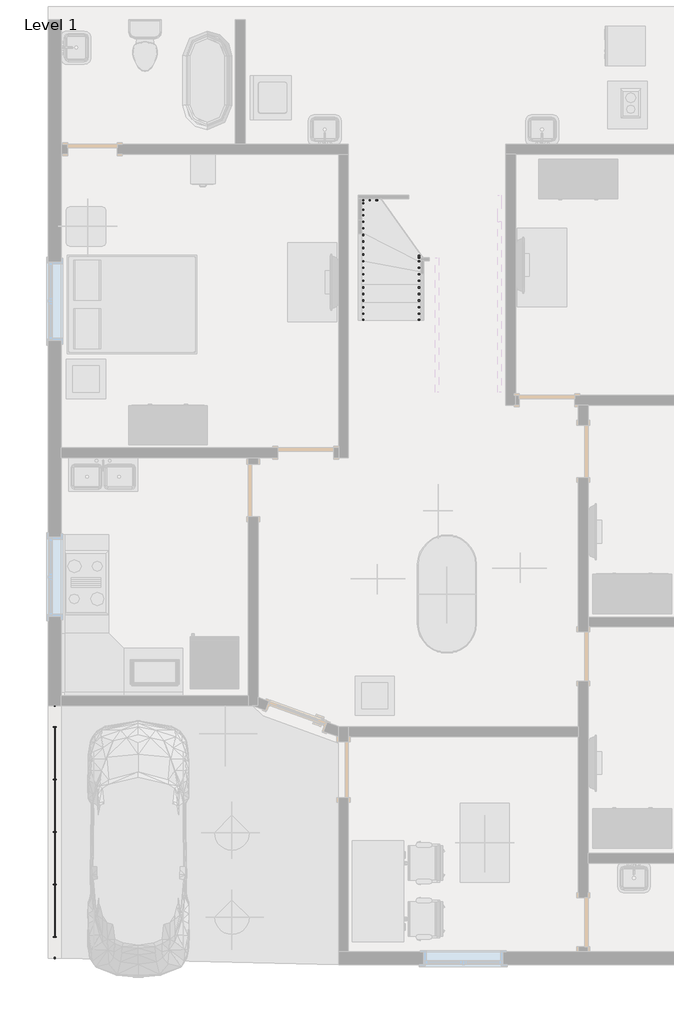
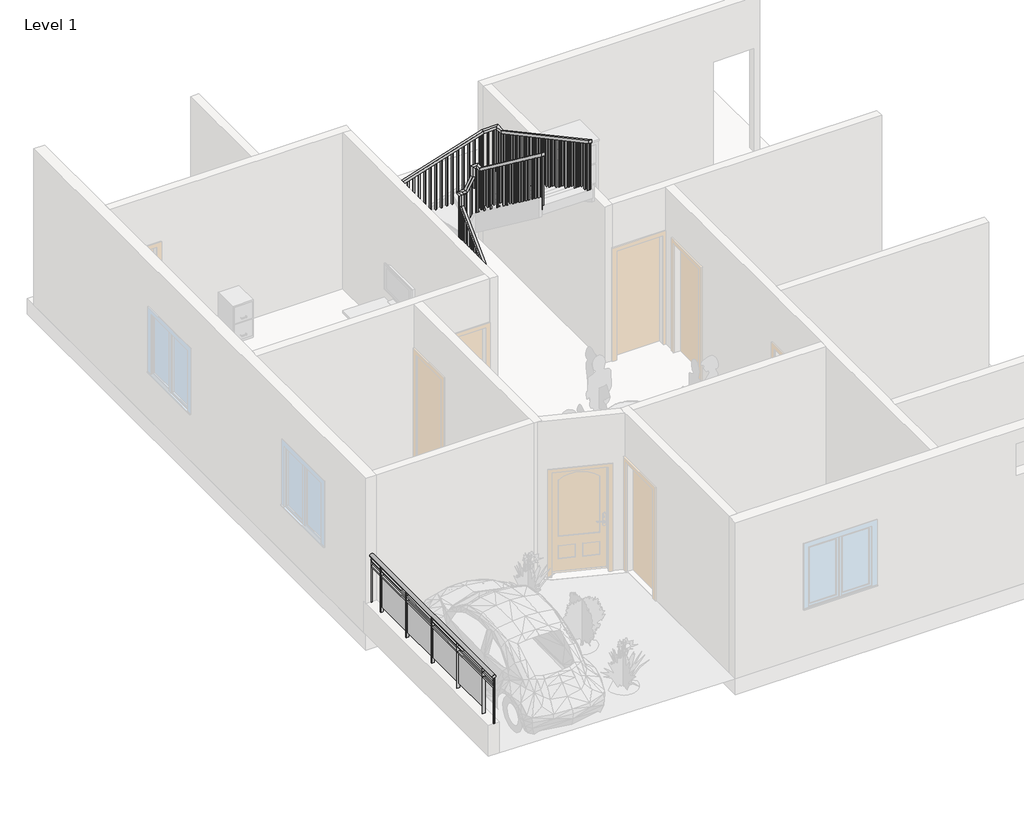
# One storey, part 2 of 3: 3 railings.
"""IFC4 building model written with IfcOpenShell, lengths in millimetres."""

from ifc_helpers import new_model, si_unit, point, frame, origin, place, context, project, spatial, polyline, ellipse_curve, trimmed, outline, extrude, faceted_brep, element, save
from ifc_brep_helpers import plane_surface, extruded_surface, advanced_brep

model = new_model("IFC4")

# Units and contexts
model_context = context("Model", 3, world=origin())
ifc_project = project(units=[si_unit("LENGTHUNIT", "METRE", prefix="MILLI")], contexts=[model_context])

# Site, building, storey
site = spatial("IfcSite", under=ifc_project)
building = spatial("IfcBuilding", under=site)
storey = spatial("IfcBuildingStorey", under=building, Name="Level 1", Elevation=0.0)

# Railings
placement = place(None, origin())
element("IfcRailing", 1, ObjectType="Glass Panel - Bottom Fill", at=placement, inside=storey, context=model_context, shape_type="SolidModel", body=[
    advanced_brep(
    [(-14836.5744419, 3106.6452409, 1524.0), (-14912.7744419, 3106.6452409, 1524.0), (-14836.5744419, -804.9547591, 1524.0), (-14912.7744419, -804.9547591, 1524.0)],
    [
        (0, 1, ellipse_curve(frame((-14874.6744419, 3106.6452409, 1524.0), z_axis=(0.0, 1.0, 0.0), x_axis=(-1.0, 0.0, 0.0)), 38.1, 28.575)),
        (1, 0, ellipse_curve(frame((-14874.6744419, 3106.6452409, 1524.0), z_axis=(0.0, 1.0, 0.0), x_axis=(-1.0, 0.0, 0.0)), 38.1, 28.575)),
        (2, 3, ellipse_curve(frame((-14874.6744419, -804.9547591, 1524.0), z_axis=(0.0, -1.0, 0.0), x_axis=(-1.0, 0.0, 0.0)), 38.1, 28.575)),
        (3, 2, ellipse_curve(frame((-14874.6744419, -804.9547591, 1524.0), z_axis=(0.0, -1.0, 0.0), x_axis=(-1.0, 0.0, 0.0)), 38.1, 28.575)),
        (0, 2),
        (3, 1),
    ],
    [
        plane_surface(frame((-14874.6744419, 3106.6452409, 1524.0), z_axis=(0.0, 1.0, 0.0), x_axis=(0.0, 0.0, -1.0))),
        plane_surface(frame((-14874.6744419, -804.9547591, 1524.0), z_axis=(0.0, -1.0, 0.0), x_axis=(0.0, 0.0, -1.0))),
        extruded_surface(trimmed(ellipse_curve(frame((-14874.6744419, -804.9547591, 1524.0), z_axis=(0.0, 1.0, 0.0), x_axis=(-1.0, 0.0, 0.0)), 38.1, 28.575), [point((-14836.5744419, -804.9547591, 1524.0))], [point((-14912.7744419, -804.9547591, 1524.0))], True, "CARTESIAN"), (0.0, 3911.6, 0.0), 3911.6),
        extruded_surface(trimmed(ellipse_curve(frame((-14874.6744419, -804.9547591, 1524.0), z_axis=(0.0, 1.0, 0.0), x_axis=(-1.0, 0.0, 0.0)), 38.1, 28.575), [point((-14912.7744419, -804.9547591, 1524.0))], [point((-14836.5744419, -804.9547591, 1524.0))], True, "CARTESIAN"), (0.0, 3911.6, 0.0), 3911.6),
    ],
    [
        (0, [[1, 2]]),
        (1, [[3, 4]]),
        (2, [[-1, 5, -4, 6]]),
        (3, [[-2, -6, -3, -5]]),
    ],
),
    extrude(outline(polyline([(-14887.3744419, 3106.6452409), (-14861.9744419, 3106.6452409), (-14861.9744419, -804.9547591), (-14887.3744419, -804.9547591), (-14887.3744419, 3106.6452409)])), frame((0.0, 0.0, 1409.7), z_axis=(0.0, 0.0, 1.0), x_axis=(1.0, 0.0, 0.0)), (0.0, 0.0, 1.0), 25.4),
    extrude(outline(polyline([(-14887.3744419, 3106.6452409), (-14861.9744419, 3106.6452409), (-14861.9744419, -804.9547591), (-14887.3744419, -804.9547591), (-14887.3744419, 3106.6452409)])), frame((0.0, 0.0, 1308.1), z_axis=(0.0, 0.0, 1.0), x_axis=(1.0, 0.0, 0.0)), (0.0, 0.0, 1.0), 25.4),
    extrude(outline(polyline([(-14900.0744419, -468.4047591), (-14849.2744419, -468.4047591), (-14849.2744419, -481.1047591), (-14900.0744419, -481.1047591), (-14900.0744419, -468.4047591)])), frame((0.0, 0.0, 609.6), z_axis=(0.0, 0.0, 1.0), x_axis=(1.0, 0.0, 0.0)), (0.0, 0.0, 1.0), 885.6788223),
    extrude(outline(polyline([(-14868.1392849, 338.0452409), (-14868.1392849, -474.7547591), (-14874.4892849, -474.7547591), (-14874.4892849, 338.0452409), (-14868.1392849, 338.0452409)])), frame((0.0, 0.0, 711.2), z_axis=(0.0, 0.0, 1.0), x_axis=(1.0, 0.0, 0.0)), (0.0, 0.0, 1.0), 596.9),
    extrude(outline(polyline([(-14900.0744419, 344.3952409), (-14849.2744419, 344.3952409), (-14849.2744419, 331.6952409), (-14900.0744419, 331.6952409), (-14900.0744419, 344.3952409)])), frame((0.0, 0.0, 609.6), z_axis=(0.0, 0.0, 1.0), x_axis=(1.0, 0.0, 0.0)), (0.0, 0.0, 1.0), 885.6788223),
    extrude(outline(polyline([(-14868.1392849, 1150.8452409), (-14868.1392849, 338.0452409), (-14874.4892849, 338.0452409), (-14874.4892849, 1150.8452409), (-14868.1392849, 1150.8452409)])), frame((0.0, 0.0, 711.2), z_axis=(0.0, 0.0, 1.0), x_axis=(1.0, 0.0, 0.0)), (0.0, 0.0, 1.0), 596.9),
    extrude(outline(polyline([(-14900.0744419, 1157.1952409), (-14849.2744419, 1157.1952409), (-14849.2744419, 1144.4952409), (-14900.0744419, 1144.4952409), (-14900.0744419, 1157.1952409)])), frame((0.0, 0.0, 609.6), z_axis=(0.0, 0.0, 1.0), x_axis=(1.0, 0.0, 0.0)), (0.0, 0.0, 1.0), 885.6788223),
    extrude(outline(polyline([(-14868.1392849, 1963.6452409), (-14868.1392849, 1150.8452409), (-14874.4892849, 1150.8452409), (-14874.4892849, 1963.6452409), (-14868.1392849, 1963.6452409)])), frame((0.0, 0.0, 711.2), z_axis=(0.0, 0.0, 1.0), x_axis=(1.0, 0.0, 0.0)), (0.0, 0.0, 1.0), 596.9),
    extrude(outline(polyline([(-14900.0744419, 1969.9952409), (-14849.2744419, 1969.9952409), (-14849.2744419, 1957.2952409), (-14900.0744419, 1957.2952409), (-14900.0744419, 1969.9952409)])), frame((0.0, 0.0, 609.6), z_axis=(0.0, 0.0, 1.0), x_axis=(1.0, 0.0, 0.0)), (0.0, 0.0, 1.0), 885.6788223),
    extrude(outline(polyline([(-14868.1392849, 2776.4452409), (-14868.1392849, 1963.6452409), (-14874.4892849, 1963.6452409), (-14874.4892849, 2776.4452409), (-14868.1392849, 2776.4452409)])), frame((0.0, 0.0, 711.2), z_axis=(0.0, 0.0, 1.0), x_axis=(1.0, 0.0, 0.0)), (0.0, 0.0, 1.0), 596.9),
    extrude(outline(polyline([(-14900.0744419, 2782.7952409), (-14849.2744419, 2782.7952409), (-14849.2744419, 2770.0952409), (-14900.0744419, 2770.0952409), (-14900.0744419, 2782.7952409)])), frame((0.0, 0.0, 609.6), z_axis=(0.0, 0.0, 1.0), x_axis=(1.0, 0.0, 0.0)), (0.0, 0.0, 1.0), 885.6788223),
    extrude(outline(polyline([(-14884.1994419, -792.2547591), (-14865.1494419, -792.2547591), (-14865.1494419, -811.3047591), (-14884.1994419, -811.3047591), (-14884.1994419, -792.2547591)])), frame((0.0, 0.0, 609.6), z_axis=(0.0, 0.0, 1.0), x_axis=(1.0, 0.0, 0.0)), (0.0, 0.0, 1.0), 885.6788223),
    extrude(outline(polyline([(-14884.1994419, 3112.9952409), (-14865.1494419, 3112.9952409), (-14865.1494419, 3093.9452409), (-14884.1994419, 3093.9452409), (-14884.1994419, 3112.9952409)])), frame((0.0, 0.0, 609.6), z_axis=(0.0, 0.0, 1.0), x_axis=(1.0, 0.0, 0.0)), (0.0, 0.0, 1.0), 885.6788223),
])
element("IfcRailing", 2, ObjectType="Handrail - Rectangular", at=placement, inside=storey, context=model_context, shape_type="SolidModel", body=[
    faceted_brep([(-9261.2744419, 9071.9135491, 1316.3704569), (-9261.2744419, 9071.9135491, 1245.0455517), (-9210.4744419, 9071.9135491, 1245.0455517), (-9210.4744419, 9071.9135491, 1316.3704569), (-9261.2744419, 9964.6452409, 2196.2028354), (-9261.2744419, 10015.4452409, 2174.9439077), (-9210.4744419, 10015.4452409, 2174.9439077), (-9210.4744419, 9964.6452409, 2196.2028354), (-9261.2744419, 9964.6452409, 2414.6281882), (-9261.2744419, 10015.4452409, 2363.8281882), (-9210.4744419, 10015.4452409, 2363.8281882), (-9210.4744419, 9964.6452409, 2414.6281882), (-9261.2744419, 10091.6452409, 2414.6281882), (-9261.2744419, 10091.6452409, 2363.8281882), (-9210.4744419, 10040.8452409, 2363.8281882), (-9210.4744419, 10040.8452409, 2414.6281882), (-9134.2744419, 10091.6452409, 2414.6281882), (-9105.1531081, 10091.6452409, 2363.8281882), (-9105.1531081, 10040.8452409, 2363.8281882), (-9134.2744419, 10040.8452409, 2414.6281882), (-9007.2744419, 10091.6452409, 2631.5051451), (-8956.4744419, 10091.6452409, 2617.7256424), (-8956.4744419, 10040.8452409, 2617.7256424), (-9007.2744419, 10040.8452409, 2631.5051451), (-9007.2744419, 10091.6452409, 2832.5574721), (-8956.4744419, 10091.6452409, 2781.7574721), (-8956.4744419, 10040.8452409, 2781.7574721), (-9007.2744419, 10040.8452409, 2832.5574721), (-8880.2744419, 10091.6452409, 2832.5574721), (-8880.2744419, 10091.6452409, 2781.7574721), (-8931.0744419, 10040.8452409, 2781.7574721), (-8931.0744419, 10040.8452409, 2832.5574721), (-8880.2744419, 9964.6452409, 2832.5574721), (-8880.2744419, 9947.7017138, 2781.7574721), (-8931.0744419, 9947.7017138, 2781.7574721), (-8931.0744419, 9964.6452409, 2832.5574721), (-8880.2744419, 7954.3135491, 4341.4410516), (-8931.0744419, 7954.3135491, 4341.4410516), (-8931.0744419, 7954.3135491, 4277.9238419), (-8880.2744419, 7954.3135491, 4277.9238419)], [[[0, 1, 2, 3]], [[1, 0, 4, 5]], [[2, 1, 5, 6]], [[3, 2, 6, 7]], [[0, 3, 7, 4]], [[5, 4, 8, 9]], [[6, 5, 9, 10]], [[7, 6, 10, 11]], [[4, 7, 11, 8]], [[9, 8, 12, 13]], [[10, 9, 13, 14]], [[11, 10, 14, 15]], [[8, 11, 15, 12]], [[13, 12, 16, 17]], [[14, 13, 17, 18]], [[15, 14, 18, 19]], [[12, 15, 19, 16]], [[17, 16, 20, 21]], [[18, 17, 21, 22]], [[19, 18, 22, 23]], [[16, 19, 23, 20]], [[21, 20, 24, 25]], [[22, 21, 25, 26]], [[23, 22, 26, 27]], [[20, 23, 27, 24]], [[25, 24, 28, 29]], [[26, 25, 29, 30]], [[27, 26, 30, 31]], [[24, 27, 31, 28]], [[29, 28, 32, 33]], [[30, 29, 33, 34]], [[31, 30, 34, 35]], [[28, 31, 35, 32]], [[36, 37, 38, 39]], [[33, 32, 36, 39]], [[34, 33, 39, 38]], [[35, 34, 38, 37]], [[32, 35, 37, 36]]]),
    extrude(outline(polyline([(7992.2736015, 4249.4323745), (8011.3236015, 4235.134121), (8011.3236015, 3217.3333333), (7992.2736015, 3217.3333333), (7992.2736015, 4249.4323745)])), frame((-8915.1994419, 0.0, 0.0), z_axis=(1.0, 0.0, 0.0), x_axis=(0.0, 1.0, 0.0)), (0.0, 0.0, 1.0), 19.05),
    extrude(outline(polyline([(8093.8736015, 4173.1750224), (8112.9236015, 4158.8767689), (8112.9236015, 3217.3333333), (8093.8736015, 3217.3333333), (8093.8736015, 4173.1750224)])), frame((-8915.1994419, 0.0, 0.0), z_axis=(1.0, 0.0, 0.0), x_axis=(0.0, 1.0, 0.0)), (0.0, 0.0, 1.0), 19.05),
    extrude(outline(polyline([(8195.4736015, 4096.9176703), (8214.5236015, 4082.6194167), (8214.5236015, 3217.3333333), (8195.4736015, 3217.3333333), (8195.4736015, 4096.9176703)])), frame((-8915.1994419, 0.0, 0.0), z_axis=(1.0, 0.0, 0.0), x_axis=(0.0, 1.0, 0.0)), (0.0, 0.0, 1.0), 19.05),
    extrude(outline(polyline([(8297.0736015, 4020.6603182), (8316.1236015, 4006.3620646), (8316.1236015, 3048.0), (8297.0736015, 3048.0), (8297.0736015, 4020.6603182)])), frame((-8915.1994419, 0.0, 0.0), z_axis=(1.0, 0.0, 0.0), x_axis=(0.0, 1.0, 0.0)), (0.0, 0.0, 1.0), 19.05),
    extrude(outline(polyline([(8398.6736015, 3944.4029661), (8417.7236015, 3930.1047125), (8417.7236015, 3048.0), (8398.6736015, 3048.0), (8398.6736015, 3944.4029661)])), frame((-8915.1994419, 0.0, 0.0), z_axis=(1.0, 0.0, 0.0), x_axis=(0.0, 1.0, 0.0)), (0.0, 0.0, 1.0), 19.05),
    extrude(outline(polyline([(8500.2736015, 3868.1456139), (8519.3236015, 3853.8473604), (8519.3236015, 3048.0), (8500.2736015, 3048.0), (8500.2736015, 3868.1456139)])), frame((-8915.1994419, 0.0, 0.0), z_axis=(1.0, 0.0, 0.0), x_axis=(0.0, 1.0, 0.0)), (0.0, 0.0, 1.0), 19.05),
    extrude(outline(polyline([(8601.8736015, 3791.8882618), (8620.9236015, 3777.5900083), (8620.9236015, 2878.6666667), (8601.8736015, 2878.6666667), (8601.8736015, 3791.8882618)])), frame((-8915.1994419, 0.0, 0.0), z_axis=(1.0, 0.0, 0.0), x_axis=(0.0, 1.0, 0.0)), (0.0, 0.0, 1.0), 19.05),
    extrude(outline(polyline([(8703.4736015, 3715.6309097), (8722.5236015, 3701.3326562), (8722.5236015, 2878.6666667), (8703.4736015, 2878.6666667), (8703.4736015, 3715.6309097)])), frame((-8915.1994419, 0.0, 0.0), z_axis=(1.0, 0.0, 0.0), x_axis=(0.0, 1.0, 0.0)), (0.0, 0.0, 1.0), 19.05),
    extrude(outline(polyline([(8805.0736015, 3639.3735576), (8824.1236015, 3625.0753041), (8824.1236015, 2709.3333333), (8805.0736015, 2709.3333333), (8805.0736015, 3639.3735576)])), frame((-8915.1994419, 0.0, 0.0), z_axis=(1.0, 0.0, 0.0), x_axis=(0.0, 1.0, 0.0)), (0.0, 0.0, 1.0), 19.05),
    extrude(outline(polyline([(8906.6736015, 3563.1162055), (8925.7236015, 3548.817952), (8925.7236015, 2709.3333333), (8906.6736015, 2709.3333333), (8906.6736015, 3563.1162055)])), frame((-8915.1994419, 0.0, 0.0), z_axis=(1.0, 0.0, 0.0), x_axis=(0.0, 1.0, 0.0)), (0.0, 0.0, 1.0), 19.05),
    extrude(outline(polyline([(9008.2736015, 3486.8588534), (9027.3236015, 3472.5605999), (9027.3236015, 2709.3333333), (9008.2736015, 2709.3333333), (9008.2736015, 3486.8588534)])), frame((-8915.1994419, 0.0, 0.0), z_axis=(1.0, 0.0, 0.0), x_axis=(0.0, 1.0, 0.0)), (0.0, 0.0, 1.0), 19.05),
    extrude(outline(polyline([(9109.8736015, 3410.6015013), (9128.9236015, 3396.3032478), (9128.9236015, 2540.0), (9109.8736015, 2540.0), (9109.8736015, 3410.6015013)])), frame((-8915.1994419, 0.0, 0.0), z_axis=(1.0, 0.0, 0.0), x_axis=(0.0, 1.0, 0.0)), (0.0, 0.0, 1.0), 19.05),
    extrude(outline(polyline([(9211.4736015, 3334.3441492), (9230.5236015, 3320.0458957), (9230.5236015, 2540.0), (9211.4736015, 2540.0), (9211.4736015, 3334.3441492)])), frame((-8915.1994419, 0.0, 0.0), z_axis=(1.0, 0.0, 0.0), x_axis=(0.0, 1.0, 0.0)), (0.0, 0.0, 1.0), 19.05),
    extrude(outline(polyline([(9313.0736015, 3258.0867971), (9332.1236015, 3243.7885436), (9332.1236015, 2370.6666667), (9313.0736015, 2370.6666667), (9313.0736015, 3258.0867971)])), frame((-8915.1994419, 0.0, 0.0), z_axis=(1.0, 0.0, 0.0), x_axis=(0.0, 1.0, 0.0)), (0.0, 0.0, 1.0), 19.05),
    extrude(outline(polyline([(9414.6736015, 3181.829445), (9433.7236015, 3167.5311915), (9433.7236015, 2370.6666667), (9414.6736015, 2370.6666667), (9414.6736015, 3181.829445)])), frame((-8915.1994419, 0.0, 0.0), z_axis=(1.0, 0.0, 0.0), x_axis=(0.0, 1.0, 0.0)), (0.0, 0.0, 1.0), 19.05),
    extrude(outline(polyline([(9516.2736015, 3105.5720929), (9535.3236015, 3091.2738394), (9535.3236015, 2370.6666667), (9516.2736015, 2370.6666667), (9516.2736015, 3105.5720929)])), frame((-8915.1994419, 0.0, 0.0), z_axis=(1.0, 0.0, 0.0), x_axis=(0.0, 1.0, 0.0)), (0.0, 0.0, 1.0), 19.05),
    extrude(outline(polyline([(9617.8736015, 3029.3147408), (9636.9236015, 3015.0164873), (9636.9236015, 2201.3333333), (9617.8736015, 2201.3333333), (9617.8736015, 3029.3147408)])), frame((-8915.1994419, 0.0, 0.0), z_axis=(1.0, 0.0, 0.0), x_axis=(0.0, 1.0, 0.0)), (0.0, 0.0, 1.0), 19.05),
    extrude(outline(polyline([(9719.4736015, 2953.0573887), (9738.5236015, 2938.7591351), (9738.5236015, 2201.3333333), (9719.4736015, 2201.3333333), (9719.4736015, 2953.0573887)])), frame((-8915.1994419, 0.0, 0.0), z_axis=(1.0, 0.0, 0.0), x_axis=(0.0, 1.0, 0.0)), (0.0, 0.0, 1.0), 19.05),
    extrude(outline(polyline([(9821.0736015, 2876.8000366), (9840.1236015, 2862.501783), (9840.1236015, 2032.0), (9821.0736015, 2032.0), (9821.0736015, 2876.8000366)])), frame((-8915.1994419, 0.0, 0.0), z_axis=(1.0, 0.0, 0.0), x_axis=(0.0, 1.0, 0.0)), (0.0, 0.0, 1.0), 19.05),
    extrude(outline(polyline([(9922.6736015, 2800.5426845), (9941.7236015, 2786.2444309), (9941.7236015, 2032.0), (9922.6736015, 2032.0), (9922.6736015, 2800.5426845)])), frame((-8915.1994419, 0.0, 0.0), z_axis=(1.0, 0.0, 0.0), x_axis=(0.0, 1.0, 0.0)), (0.0, 0.0, 1.0), 19.05),
    extrude(outline(polyline([(2531.4693239, -9006.9848908), (2498.9377803, -9026.0348908), (1524.0, -9026.0348908), (1524.0, -9006.9848908), (2531.4693239, -9006.9848908)])), frame((0.0, 10056.7202409, 0.0), z_axis=(0.0, 1.0, 0.0), x_axis=(0.0, 0.0, 1.0)), (0.0, 0.0, 1.0), 19.05),
    extrude(outline(polyline([(2357.9677583, -9108.5848908), (2325.4362148, -9127.6348908), (1524.0, -9127.6348908), (1524.0, -9108.5848908), (2357.9677583, -9108.5848908)])), frame((0.0, 10056.7202409, 0.0), z_axis=(0.0, 1.0, 0.0), x_axis=(0.0, 0.0, 1.0)), (0.0, 0.0, 1.0), 19.05),
    extrude(outline(polyline([(9976.7885491, 2136.8457765), (9995.8385491, 2155.620518), (9995.8385491, 1185.3333333), (9976.7885491, 1185.3333333), (9976.7885491, 2136.8457765)])), frame((-9245.3994419, 0.0, 0.0), z_axis=(1.0, 0.0, 0.0), x_axis=(0.0, 1.0, 0.0)), (0.0, 0.0, 1.0), 19.05),
    extrude(outline(polyline([(9875.1885491, 2036.7138214), (9894.2385491, 2055.488563), (9894.2385491, 1016.0), (9875.1885491, 1016.0), (9875.1885491, 2036.7138214)])), frame((-9245.3994419, 0.0, 0.0), z_axis=(1.0, 0.0, 0.0), x_axis=(0.0, 1.0, 0.0)), (0.0, 0.0, 1.0), 19.05),
    extrude(outline(polyline([(9773.5885491, 1936.5818663), (9792.6385491, 1955.3566079), (9792.6385491, 846.6666667), (9773.5885491, 846.6666667), (9773.5885491, 1936.5818663)])), frame((-9245.3994419, 0.0, 0.0), z_axis=(1.0, 0.0, 0.0), x_axis=(0.0, 1.0, 0.0)), (0.0, 0.0, 1.0), 19.05),
    extrude(outline(polyline([(9671.9885491, 1836.4499113), (9691.0385491, 1855.2246528), (9691.0385491, 846.6666667), (9671.9885491, 846.6666667), (9671.9885491, 1836.4499113)])), frame((-9245.3994419, 0.0, 0.0), z_axis=(1.0, 0.0, 0.0), x_axis=(0.0, 1.0, 0.0)), (0.0, 0.0, 1.0), 19.05),
    extrude(outline(polyline([(9570.3885491, 1736.3179562), (9589.4385491, 1755.0926978), (9589.4385491, 677.3333333), (9570.3885491, 677.3333333), (9570.3885491, 1736.3179562)])), frame((-9245.3994419, 0.0, 0.0), z_axis=(1.0, 0.0, 0.0), x_axis=(0.0, 1.0, 0.0)), (0.0, 0.0, 1.0), 19.05),
    extrude(outline(polyline([(9468.7885491, 1636.1860011), (9487.8385491, 1654.9607427), (9487.8385491, 677.3333333), (9468.7885491, 677.3333333), (9468.7885491, 1636.1860011)])), frame((-9245.3994419, 0.0, 0.0), z_axis=(1.0, 0.0, 0.0), x_axis=(0.0, 1.0, 0.0)), (0.0, 0.0, 1.0), 19.05),
    extrude(outline(polyline([(9367.1885491, 1536.0540461), (9386.2385491, 1554.8287877), (9386.2385491, 677.3333333), (9367.1885491, 677.3333333), (9367.1885491, 1536.0540461)])), frame((-9245.3994419, 0.0, 0.0), z_axis=(1.0, 0.0, 0.0), x_axis=(0.0, 1.0, 0.0)), (0.0, 0.0, 1.0), 19.05),
    extrude(outline(polyline([(9265.5885491, 1435.922091), (9284.6385491, 1454.6968326), (9284.6385491, 508.0), (9265.5885491, 508.0), (9265.5885491, 1435.922091)])), frame((-9245.3994419, 0.0, 0.0), z_axis=(1.0, 0.0, 0.0), x_axis=(0.0, 1.0, 0.0)), (0.0, 0.0, 1.0), 19.05),
    extrude(outline(polyline([(9163.9885491, 1335.790136), (9183.0385491, 1354.5648775), (9183.0385491, 508.0), (9163.9885491, 508.0), (9163.9885491, 1335.790136)])), frame((-9245.3994419, 0.0, 0.0), z_axis=(1.0, 0.0, 0.0), x_axis=(0.0, 1.0, 0.0)), (0.0, 0.0, 1.0), 19.05),
    extrude(outline(polyline([(-8915.1994419, 10043.3236015), (-8896.1494419, 10043.3236015), (-8896.1494419, 10024.2736015), (-8915.1994419, 10024.2736015), (-8915.1994419, 10043.3236015)])), frame((0.0, 0.0, 1862.6666667), z_axis=(0.0, 0.0, 1.0), x_axis=(1.0, 0.0, 0.0)), (0.0, 0.0, 1.0), 919.0908055),
    extrude(outline(polyline([(-8915.1994419, 10056.7202409), (-8915.1994419, 10075.7702409), (-8896.1494419, 10075.7702409), (-8896.1494419, 10056.7202409), (-8915.1994419, 10056.7202409)])), frame((0.0, 0.0, 1862.6666667), z_axis=(0.0, 0.0, 1.0), x_axis=(1.0, 0.0, 0.0)), (0.0, 0.0, 1.0), 919.0908055),
    extrude(outline(polyline([(-8929.4603784, 10056.7202409), (-8929.4603784, 10075.7702409), (-8910.4103784, 10075.7702409), (-8910.4103784, 10056.7202409), (-8929.4603784, 10056.7202409)])), frame((0.0, 0.0, 1693.3333333), z_axis=(0.0, 0.0, 1.0), x_axis=(1.0, 0.0, 0.0)), (0.0, 0.0, 1.0), 1088.4241388),
    extrude(outline(polyline([(-9229.2348908, 10056.7202409), (-9229.2348908, 10075.7702409), (-9210.1848908, 10075.7702409), (-9210.1848908, 10056.7202409), (-9229.2348908, 10056.7202409)])), frame((0.0, 0.0, 1354.6666667), z_axis=(0.0, 0.0, 1.0), x_axis=(1.0, 0.0, 0.0)), (0.0, 0.0, 1.0), 1009.1615215),
    extrude(outline(polyline([(-9226.3494419, 10056.7202409), (-9245.3994419, 10056.7202409), (-9245.3994419, 10075.7702409), (-9226.3494419, 10075.7702409), (-9226.3494419, 10056.7202409)])), frame((0.0, 0.0, 1185.3333333), z_axis=(0.0, 0.0, 1.0), x_axis=(1.0, 0.0, 0.0)), (0.0, 0.0, 1.0), 1178.4948549),
    extrude(outline(polyline([(-9226.3494419, 10028.7114507), (-9245.3994419, 10028.7114507), (-9245.3994419, 10047.7614507), (-9226.3494419, 10047.7614507), (-9226.3494419, 10028.7114507)])), frame((0.0, 0.0, 1185.3333333), z_axis=(0.0, 0.0, 1.0), x_axis=(1.0, 0.0, 0.0)), (0.0, 0.0, 1.0), 1178.4948549),
    extrude(outline(polyline([(7954.3135491, 4277.9238419), (7973.3635491, 4263.6255883), (7973.3635491, 3217.3333333), (7954.3135491, 3217.3333333), (7954.3135491, 4277.9238419)])), frame((-8915.1994419, 0.0, 0.0), z_axis=(1.0, 0.0, 0.0), x_axis=(0.0, 1.0, 0.0)), (0.0, 0.0, 1.0), 19.05),
    extrude(outline(polyline([(9071.9135491, 1245.0455517), (9090.9635491, 1263.8202933), (9090.9635491, 508.0), (9071.9135491, 508.0), (9071.9135491, 1245.0455517)])), frame((-9245.3994419, 0.0, 0.0), z_axis=(1.0, 0.0, 0.0), x_axis=(0.0, 1.0, 0.0)), (0.0, 0.0, 1.0), 19.05),
])
element("IfcRailing", 3, ObjectType="Handrail - Rectangular", at=placement, inside=storey, context=model_context, shape_type="SolidModel", body=[
    faceted_brep([(-10124.8744419, 9071.9135491, 1460.80748), (-10124.8744419, 9071.9135491, 1404.7066442), (-10074.0744419, 9071.9135491, 1404.7066442), (-10074.0744419, 9071.9135491, 1460.80748), (-10124.8744419, 10782.1225833, 2262.2053941), (-10124.8744419, 10793.434738, 2211.4053941), (-10074.0744419, 10793.434738, 2211.4053941), (-10074.0744419, 10782.1225833, 2262.2053941), (-10124.8744419, 10955.2452409, 2262.2053941), (-10124.8744419, 10955.2452409, 2211.4053941), (-10074.0744419, 10904.4452409, 2211.4053941), (-10074.0744419, 10904.4452409, 2262.2053941), (-9883.744249, 10955.2452409, 2262.2053941), (-9875.7936729, 10955.2452409, 2211.4053941), (-9875.7936729, 10904.4452409, 2211.4053941), (-9883.744249, 10904.4452409, 2262.2053941), (-8311.5661181, 10955.2452409, 2766.6772507), (-8303.6155419, 10955.2452409, 2715.8772507), (-8303.6155419, 10904.4452409, 2715.8772507), (-8311.5661181, 10904.4452409, 2766.6772507), (-8016.6744419, 10955.2452409, 2766.6772507), (-8016.6744419, 10955.2452409, 2715.8772507), (-8067.4744419, 10904.4452409, 2715.8772507), (-8067.4744419, 10904.4452409, 2766.6772507), (-8016.6744419, 10769.2266151, 2766.6772507), (-8016.6744419, 10756.4208607, 2715.8772507), (-8067.4744419, 10756.4208607, 2715.8772507), (-8067.4744419, 10769.2266151, 2766.6772507), (-8016.6744419, 7954.3135491, 4282.1552241), (-8067.4744419, 7954.3135491, 4282.1552241), (-8067.4744419, 7954.3135491, 4224.46093), (-8016.6744419, 7954.3135491, 4224.46093)], [[[0, 1, 2, 3]], [[1, 0, 4, 5]], [[2, 1, 5, 6]], [[3, 2, 6, 7]], [[0, 3, 7, 4]], [[5, 4, 8, 9]], [[6, 5, 9, 10]], [[7, 6, 10, 11]], [[4, 7, 11, 8]], [[9, 8, 12, 13]], [[10, 9, 13, 14]], [[11, 10, 14, 15]], [[8, 11, 15, 12]], [[13, 12, 16, 17]], [[14, 13, 17, 18]], [[15, 14, 18, 19]], [[12, 15, 19, 16]], [[17, 16, 20, 21]], [[18, 17, 21, 22]], [[19, 18, 22, 23]], [[16, 19, 23, 20]], [[21, 20, 24, 25]], [[22, 21, 25, 26]], [[23, 22, 26, 27]], [[20, 23, 27, 24]], [[28, 29, 30, 31]], [[25, 24, 28, 31]], [[26, 25, 31, 30]], [[27, 26, 30, 29]], [[24, 27, 29, 28]]]),
    extrude(outline(polyline([(8035.5516151, 4180.7244106), (8035.5516151, 3217.3333333), (8016.5016151, 3217.3333333), (8016.5016151, 4190.9804487), (8035.5516151, 4180.7244106)])), frame((-8051.5994419, 0.0, 0.0), z_axis=(1.0, 0.0, 0.0), x_axis=(0.0, 1.0, 0.0)), (0.0, 0.0, 1.0), 19.05),
    extrude(outline(polyline([(8137.1516151, 4126.0255413), (8137.1516151, 3217.3333333), (8118.1016151, 3217.3333333), (8118.1016151, 4136.2815793), (8137.1516151, 4126.0255413)])), frame((-8051.5994419, 0.0, 0.0), z_axis=(1.0, 0.0, 0.0), x_axis=(0.0, 1.0, 0.0)), (0.0, 0.0, 1.0), 19.05),
    extrude(outline(polyline([(8238.7516151, 4071.3266719), (8238.7516151, 3217.3333333), (8219.7016151, 3217.3333333), (8219.7016151, 4081.5827099), (8238.7516151, 4071.3266719)])), frame((-8051.5994419, 0.0, 0.0), z_axis=(1.0, 0.0, 0.0), x_axis=(0.0, 1.0, 0.0)), (0.0, 0.0, 1.0), 19.05),
    extrude(outline(polyline([(8340.3516151, 4016.6278025), (8340.3516151, 3048.0), (8321.3016151, 3048.0), (8321.3016151, 4026.8838405), (8340.3516151, 4016.6278025)])), frame((-8051.5994419, 0.0, 0.0), z_axis=(1.0, 0.0, 0.0), x_axis=(0.0, 1.0, 0.0)), (0.0, 0.0, 1.0), 19.05),
    extrude(outline(polyline([(8441.9516151, 3961.9289332), (8441.9516151, 3048.0), (8422.9016151, 3048.0), (8422.9016151, 3972.1849712), (8441.9516151, 3961.9289332)])), frame((-8051.5994419, 0.0, 0.0), z_axis=(1.0, 0.0, 0.0), x_axis=(0.0, 1.0, 0.0)), (0.0, 0.0, 1.0), 19.05),
    extrude(outline(polyline([(8543.5516151, 3907.2300638), (8543.5516151, 2878.6666667), (8524.5016151, 2878.6666667), (8524.5016151, 3917.4861018), (8543.5516151, 3907.2300638)])), frame((-8051.5994419, 0.0, 0.0), z_axis=(1.0, 0.0, 0.0), x_axis=(0.0, 1.0, 0.0)), (0.0, 0.0, 1.0), 19.05),
    extrude(outline(polyline([(8645.1516151, 3852.5311944), (8645.1516151, 2878.6666667), (8626.1016151, 2878.6666667), (8626.1016151, 3862.7872324), (8645.1516151, 3852.5311944)])), frame((-8051.5994419, 0.0, 0.0), z_axis=(1.0, 0.0, 0.0), x_axis=(0.0, 1.0, 0.0)), (0.0, 0.0, 1.0), 19.05),
    extrude(outline(polyline([(8746.7516151, 3797.832325), (8746.7516151, 2878.6666667), (8727.7016151, 2878.6666667), (8727.7016151, 3808.088363), (8746.7516151, 3797.832325)])), frame((-8051.5994419, 0.0, 0.0), z_axis=(1.0, 0.0, 0.0), x_axis=(0.0, 1.0, 0.0)), (0.0, 0.0, 1.0), 19.05),
    extrude(outline(polyline([(8848.3516151, 3743.1334557), (8848.3516151, 2709.3333333), (8829.3016151, 2709.3333333), (8829.3016151, 3753.3894937), (8848.3516151, 3743.1334557)])), frame((-8051.5994419, 0.0, 0.0), z_axis=(1.0, 0.0, 0.0), x_axis=(0.0, 1.0, 0.0)), (0.0, 0.0, 1.0), 19.05),
    extrude(outline(polyline([(8949.9516151, 3688.4345863), (8949.9516151, 2709.3333333), (8930.9016151, 2709.3333333), (8930.9016151, 3698.6906243), (8949.9516151, 3688.4345863)])), frame((-8051.5994419, 0.0, 0.0), z_axis=(1.0, 0.0, 0.0), x_axis=(0.0, 1.0, 0.0)), (0.0, 0.0, 1.0), 19.05),
    extrude(outline(polyline([(9051.5516151, 3633.7357169), (9051.5516151, 2709.3333333), (9032.5016151, 2709.3333333), (9032.5016151, 3643.9917549), (9051.5516151, 3633.7357169)])), frame((-8051.5994419, 0.0, 0.0), z_axis=(1.0, 0.0, 0.0), x_axis=(0.0, 1.0, 0.0)), (0.0, 0.0, 1.0), 19.05),
    extrude(outline(polyline([(9153.1516151, 3579.0368475), (9153.1516151, 2540.0), (9134.1016151, 2540.0), (9134.1016151, 3589.2928855), (9153.1516151, 3579.0368475)])), frame((-8051.5994419, 0.0, 0.0), z_axis=(1.0, 0.0, 0.0), x_axis=(0.0, 1.0, 0.0)), (0.0, 0.0, 1.0), 19.05),
    extrude(outline(polyline([(9254.7516151, 3524.3379782), (9254.7516151, 2540.0), (9235.7016151, 2540.0), (9235.7016151, 3534.5940162), (9254.7516151, 3524.3379782)])), frame((-8051.5994419, 0.0, 0.0), z_axis=(1.0, 0.0, 0.0), x_axis=(0.0, 1.0, 0.0)), (0.0, 0.0, 1.0), 19.05),
    extrude(outline(polyline([(9356.3516151, 3469.6391088), (9356.3516151, 2540.0), (9337.3016151, 2540.0), (9337.3016151, 3479.8951468), (9356.3516151, 3469.6391088)])), frame((-8051.5994419, 0.0, 0.0), z_axis=(1.0, 0.0, 0.0), x_axis=(0.0, 1.0, 0.0)), (0.0, 0.0, 1.0), 19.05),
    extrude(outline(polyline([(9457.9516151, 3414.9402394), (9457.9516151, 2370.6666667), (9438.9016151, 2370.6666667), (9438.9016151, 3425.1962774), (9457.9516151, 3414.9402394)])), frame((-8051.5994419, 0.0, 0.0), z_axis=(1.0, 0.0, 0.0), x_axis=(0.0, 1.0, 0.0)), (0.0, 0.0, 1.0), 19.05),
    extrude(outline(polyline([(9559.5516151, 3360.24137), (9559.5516151, 2370.6666667), (9540.5016151, 2370.6666667), (9540.5016151, 3370.497408), (9559.5516151, 3360.24137)])), frame((-8051.5994419, 0.0, 0.0), z_axis=(1.0, 0.0, 0.0), x_axis=(0.0, 1.0, 0.0)), (0.0, 0.0, 1.0), 19.05),
    extrude(outline(polyline([(9661.1516151, 3305.5425007), (9661.1516151, 2370.6666667), (9642.1016151, 2370.6666667), (9642.1016151, 3315.7985387), (9661.1516151, 3305.5425007)])), frame((-8051.5994419, 0.0, 0.0), z_axis=(1.0, 0.0, 0.0), x_axis=(0.0, 1.0, 0.0)), (0.0, 0.0, 1.0), 19.05),
    extrude(outline(polyline([(9762.7516151, 3250.8436313), (9762.7516151, 2201.3333333), (9743.7016151, 2201.3333333), (9743.7016151, 3261.0996693), (9762.7516151, 3250.8436313)])), frame((-8051.5994419, 0.0, 0.0), z_axis=(1.0, 0.0, 0.0), x_axis=(0.0, 1.0, 0.0)), (0.0, 0.0, 1.0), 19.05),
    extrude(outline(polyline([(9864.3516151, 3196.1447619), (9864.3516151, 2201.3333333), (9845.3016151, 2201.3333333), (9845.3016151, 3206.4007999), (9864.3516151, 3196.1447619)])), frame((-8051.5994419, 0.0, 0.0), z_axis=(1.0, 0.0, 0.0), x_axis=(0.0, 1.0, 0.0)), (0.0, 0.0, 1.0), 19.05),
    extrude(outline(polyline([(9965.9516151, 3141.4458925), (9965.9516151, 2201.3333333), (9946.9016151, 2201.3333333), (9946.9016151, 3151.7019305), (9965.9516151, 3141.4458925)])), frame((-8051.5994419, 0.0, 0.0), z_axis=(1.0, 0.0, 0.0), x_axis=(0.0, 1.0, 0.0)), (0.0, 0.0, 1.0), 19.05),
    extrude(outline(polyline([(10067.5516151, 3086.7470232), (10067.5516151, 2032.0), (10048.5016151, 2032.0), (10048.5016151, 3097.0030612), (10067.5516151, 3086.7470232)])), frame((-8051.5994419, 0.0, 0.0), z_axis=(1.0, 0.0, 0.0), x_axis=(0.0, 1.0, 0.0)), (0.0, 0.0, 1.0), 19.05),
    extrude(outline(polyline([(10169.1516151, 3032.0481538), (10169.1516151, 2032.0), (10150.1016151, 2032.0), (10150.1016151, 3042.3041918), (10169.1516151, 3032.0481538)])), frame((-8051.5994419, 0.0, 0.0), z_axis=(1.0, 0.0, 0.0), x_axis=(0.0, 1.0, 0.0)), (0.0, 0.0, 1.0), 19.05),
    extrude(outline(polyline([(10270.7516151, 2977.3492844), (10270.7516151, 2032.0), (10251.7016151, 2032.0), (10251.7016151, 2987.6053224), (10270.7516151, 2977.3492844)])), frame((-8051.5994419, 0.0, 0.0), z_axis=(1.0, 0.0, 0.0), x_axis=(0.0, 1.0, 0.0)), (0.0, 0.0, 1.0), 19.05),
    extrude(outline(polyline([(10372.3516151, 2922.650415), (10372.3516151, 2032.0), (10353.3016151, 2032.0), (10353.3016151, 2932.906453), (10372.3516151, 2922.650415)])), frame((-8051.5994419, 0.0, 0.0), z_axis=(1.0, 0.0, 0.0), x_axis=(0.0, 1.0, 0.0)), (0.0, 0.0, 1.0), 19.05),
    extrude(outline(polyline([(10473.9516151, 2867.9515457), (10473.9516151, 1862.6666667), (10454.9016151, 1862.6666667), (10454.9016151, 2878.2075837), (10473.9516151, 2867.9515457)])), frame((-8051.5994419, 0.0, 0.0), z_axis=(1.0, 0.0, 0.0), x_axis=(0.0, 1.0, 0.0)), (0.0, 0.0, 1.0), 19.05),
    extrude(outline(polyline([(10575.5516151, 2813.2526763), (10575.5516151, 1862.6666667), (10556.5016151, 1862.6666667), (10556.5016151, 2823.5087143), (10575.5516151, 2813.2526763)])), frame((-8051.5994419, 0.0, 0.0), z_axis=(1.0, 0.0, 0.0), x_axis=(0.0, 1.0, 0.0)), (0.0, 0.0, 1.0), 19.05),
    extrude(outline(polyline([(10677.1516151, 2758.5538069), (10677.1516151, 1862.6666667), (10658.1016151, 1862.6666667), (10658.1016151, 2768.8098449), (10677.1516151, 2758.5538069)])), frame((-8051.5994419, 0.0, 0.0), z_axis=(1.0, 0.0, 0.0), x_axis=(0.0, 1.0, 0.0)), (0.0, 0.0, 1.0), 19.05),
    extrude(outline(polyline([(-8032.5494419, 10837.7702409), (-8032.5494419, 10818.7202409), (-8051.5994419, 10818.7202409), (-8051.5994419, 10837.7702409), (-8032.5494419, 10837.7702409)])), frame((0.0, 0.0, 1862.6666667), z_axis=(0.0, 0.0, 1.0), x_axis=(1.0, 0.0, 0.0)), (0.0, 0.0, 1.0), 853.210584),
    extrude(outline(polyline([(-8117.8911181, 10939.3702409), (-8098.8411181, 10939.3702409), (-8098.8411181, 10920.3202409), (-8117.8911181, 10920.3202409), (-8117.8911181, 10939.3702409)])), frame((0.0, 0.0, 1862.6666667), z_axis=(0.0, 0.0, 1.0), x_axis=(1.0, 0.0, 0.0)), (0.0, 0.0, 1.0), 853.210584),
    extrude(outline(polyline([(-8219.4911181, 10939.3702409), (-8200.4411181, 10939.3702409), (-8200.4411181, 10920.3202409), (-8219.4911181, 10920.3202409), (-8219.4911181, 10939.3702409)])), frame((0.0, 0.0, 1862.6666667), z_axis=(0.0, 0.0, 1.0), x_axis=(1.0, 0.0, 0.0)), (0.0, 0.0, 1.0), 853.210584),
    extrude(outline(polyline([(2694.8106509, -8369.269249), (1693.3333333, -8369.269249), (1693.3333333, -8350.219249), (2700.9233099, -8350.219249), (2694.8106509, -8369.269249)])), frame((0.0, 10920.3202409, 0.0), z_axis=(0.0, 1.0, 0.0), x_axis=(0.0, 0.0, 1.0)), (0.0, 0.0, 1.0), 19.05),
    extrude(outline(polyline([(2662.2098027, -8470.869249), (1693.3333333, -8470.869249), (1693.3333333, -8451.819249), (2668.3224617, -8451.819249), (2662.2098027, -8470.869249)])), frame((0.0, 10920.3202409, 0.0), z_axis=(0.0, 1.0, 0.0), x_axis=(0.0, 0.0, 1.0)), (0.0, 0.0, 1.0), 19.05),
    extrude(outline(polyline([(2629.6089544, -8572.469249), (1693.3333333, -8572.469249), (1693.3333333, -8553.419249), (2635.7216135, -8553.419249), (2629.6089544, -8572.469249)])), frame((0.0, 10920.3202409, 0.0), z_axis=(0.0, 1.0, 0.0), x_axis=(0.0, 0.0, 1.0)), (0.0, 0.0, 1.0), 19.05),
    extrude(outline(polyline([(2597.0081062, -8674.069249), (1693.3333333, -8674.069249), (1693.3333333, -8655.019249), (2603.1207653, -8655.019249), (2597.0081062, -8674.069249)])), frame((0.0, 10920.3202409, 0.0), z_axis=(0.0, 1.0, 0.0), x_axis=(0.0, 0.0, 1.0)), (0.0, 0.0, 1.0), 19.05),
    extrude(outline(polyline([(2564.407258, -8775.669249), (1693.3333333, -8775.669249), (1693.3333333, -8756.619249), (2570.519917, -8756.619249), (2564.407258, -8775.669249)])), frame((0.0, 10920.3202409, 0.0), z_axis=(0.0, 1.0, 0.0), x_axis=(0.0, 0.0, 1.0)), (0.0, 0.0, 1.0), 19.05),
    extrude(outline(polyline([(2531.8064098, -8877.269249), (1524.0, -8877.269249), (1524.0, -8858.219249), (2537.9190688, -8858.219249), (2531.8064098, -8877.269249)])), frame((0.0, 10920.3202409, 0.0), z_axis=(0.0, 1.0, 0.0), x_axis=(0.0, 0.0, 1.0)), (0.0, 0.0, 1.0), 19.05),
    extrude(outline(polyline([(2499.2055615, -8978.869249), (1524.0, -8978.869249), (1524.0, -8959.819249), (2505.3182206, -8959.819249), (2499.2055615, -8978.869249)])), frame((0.0, 10920.3202409, 0.0), z_axis=(0.0, 1.0, 0.0), x_axis=(0.0, 0.0, 1.0)), (0.0, 0.0, 1.0), 19.05),
    extrude(outline(polyline([(2466.6047133, -9080.469249), (1524.0, -9080.469249), (1524.0, -9061.419249), (2472.7173724, -9061.419249), (2466.6047133, -9080.469249)])), frame((0.0, 10920.3202409, 0.0), z_axis=(0.0, 1.0, 0.0), x_axis=(0.0, 0.0, 1.0)), (0.0, 0.0, 1.0), 19.05),
    extrude(outline(polyline([(2434.0038651, -9182.069249), (1524.0, -9182.069249), (1524.0, -9163.019249), (2440.1165241, -9163.019249), (2434.0038651, -9182.069249)])), frame((0.0, 10920.3202409, 0.0), z_axis=(0.0, 1.0, 0.0), x_axis=(0.0, 0.0, 1.0)), (0.0, 0.0, 1.0), 19.05),
    extrude(outline(polyline([(2401.4030169, -9283.669249), (1524.0, -9283.669249), (1524.0, -9264.619249), (2407.5156759, -9264.619249), (2401.4030169, -9283.669249)])), frame((0.0, 10920.3202409, 0.0), z_axis=(0.0, 1.0, 0.0), x_axis=(0.0, 0.0, 1.0)), (0.0, 0.0, 1.0), 19.05),
    extrude(outline(polyline([(2368.8021686, -9385.269249), (1354.6666667, -9385.269249), (1354.6666667, -9366.219249), (2374.9148277, -9366.219249), (2368.8021686, -9385.269249)])), frame((0.0, 10920.3202409, 0.0), z_axis=(0.0, 1.0, 0.0), x_axis=(0.0, 0.0, 1.0)), (0.0, 0.0, 1.0), 19.05),
    extrude(outline(polyline([(2336.2013204, -9486.869249), (1354.6666667, -9486.869249), (1354.6666667, -9467.819249), (2342.3139794, -9467.819249), (2336.2013204, -9486.869249)])), frame((0.0, 10920.3202409, 0.0), z_axis=(0.0, 1.0, 0.0), x_axis=(0.0, 0.0, 1.0)), (0.0, 0.0, 1.0), 19.05),
    extrude(outline(polyline([(2303.6004722, -9588.469249), (1354.6666667, -9588.469249), (1354.6666667, -9569.419249), (2309.7131312, -9569.419249), (2303.6004722, -9588.469249)])), frame((0.0, 10920.3202409, 0.0), z_axis=(0.0, 1.0, 0.0), x_axis=(0.0, 0.0, 1.0)), (0.0, 0.0, 1.0), 19.05),
    extrude(outline(polyline([(2270.999624, -9690.069249), (1354.6666667, -9690.069249), (1354.6666667, -9671.019249), (2277.112283, -9671.019249), (2270.999624, -9690.069249)])), frame((0.0, 10920.3202409, 0.0), z_axis=(0.0, 1.0, 0.0), x_axis=(0.0, 0.0, 1.0)), (0.0, 0.0, 1.0), 19.05),
    extrude(outline(polyline([(2238.3987757, -9791.669249), (1354.6666667, -9791.669249), (1354.6666667, -9772.619249), (2244.5114348, -9772.619249), (2238.3987757, -9791.669249)])), frame((0.0, 10920.3202409, 0.0), z_axis=(0.0, 1.0, 0.0), x_axis=(0.0, 0.0, 1.0)), (0.0, 0.0, 1.0), 19.05),
    extrude(outline(polyline([(-9905.7994419, 10939.3702409), (-9886.7494419, 10939.3702409), (-9886.7494419, 10920.3202409), (-9905.7994419, 10920.3202409), (-9905.7994419, 10939.3702409)])), frame((0.0, 0.0, 1185.3333333), z_axis=(0.0, 0.0, 1.0), x_axis=(1.0, 0.0, 0.0)), (0.0, 0.0, 1.0), 1026.0720608),
    extrude(outline(polyline([(-10007.3994419, 10939.3702409), (-9988.3494419, 10939.3702409), (-9988.3494419, 10920.3202409), (-10007.3994419, 10920.3202409), (-10007.3994419, 10939.3702409)])), frame((0.0, 0.0, 1185.3333333), z_axis=(0.0, 0.0, 1.0), x_axis=(1.0, 0.0, 0.0)), (0.0, 0.0, 1.0), 1026.0720608),
    extrude(outline(polyline([(-10108.9994419, 10874.1975833), (-10108.9994419, 10893.2475833), (-10089.9494419, 10893.2475833), (-10089.9494419, 10874.1975833), (-10108.9994419, 10874.1975833)])), frame((0.0, 0.0, 1185.3333333), z_axis=(0.0, 0.0, 1.0), x_axis=(1.0, 0.0, 0.0)), (0.0, 0.0, 1.0), 1026.0720608),
    extrude(outline(polyline([(10707.0385491, 2170.9204451), (10707.0385491, 1185.3333333), (10687.9885491, 1185.3333333), (10687.9885491, 2161.9936823), (10707.0385491, 2170.9204451)])), frame((-10108.9994419, 0.0, 0.0), z_axis=(1.0, 0.0, 0.0), x_axis=(0.0, 1.0, 0.0)), (0.0, 0.0, 1.0), 19.05),
    extrude(outline(polyline([(10605.4385491, 2123.3110438), (10605.4385491, 1185.3333333), (10586.3885491, 1185.3333333), (10586.3885491, 2114.3842811), (10605.4385491, 2123.3110438)])), frame((-10108.9994419, 0.0, 0.0), z_axis=(1.0, 0.0, 0.0), x_axis=(0.0, 1.0, 0.0)), (0.0, 0.0, 1.0), 19.05),
    extrude(outline(polyline([(10503.8385491, 2075.7016426), (10503.8385491, 1185.3333333), (10484.7885491, 1185.3333333), (10484.7885491, 2066.7748799), (10503.8385491, 2075.7016426)])), frame((-10108.9994419, 0.0, 0.0), z_axis=(1.0, 0.0, 0.0), x_axis=(0.0, 1.0, 0.0)), (0.0, 0.0, 1.0), 19.05),
    extrude(outline(polyline([(10402.2385491, 2028.0922414), (10402.2385491, 1016.0), (10383.1885491, 1016.0), (10383.1885491, 2019.1654787), (10402.2385491, 2028.0922414)])), frame((-10108.9994419, 0.0, 0.0), z_axis=(1.0, 0.0, 0.0), x_axis=(0.0, 1.0, 0.0)), (0.0, 0.0, 1.0), 19.05),
    extrude(outline(polyline([(10300.6385491, 1980.4828402), (10300.6385491, 1016.0), (10281.5885491, 1016.0), (10281.5885491, 1971.5560775), (10300.6385491, 1980.4828402)])), frame((-10108.9994419, 0.0, 0.0), z_axis=(1.0, 0.0, 0.0), x_axis=(0.0, 1.0, 0.0)), (0.0, 0.0, 1.0), 19.05),
    extrude(outline(polyline([(10199.0385491, 1932.873439), (10199.0385491, 1016.0), (10179.9885491, 1016.0), (10179.9885491, 1923.9466763), (10199.0385491, 1932.873439)])), frame((-10108.9994419, 0.0, 0.0), z_axis=(1.0, 0.0, 0.0), x_axis=(0.0, 1.0, 0.0)), (0.0, 0.0, 1.0), 19.05),
    extrude(outline(polyline([(10097.4385491, 1885.2640378), (10097.4385491, 1016.0), (10078.3885491, 1016.0), (10078.3885491, 1876.337275), (10097.4385491, 1885.2640378)])), frame((-10108.9994419, 0.0, 0.0), z_axis=(1.0, 0.0, 0.0), x_axis=(0.0, 1.0, 0.0)), (0.0, 0.0, 1.0), 19.05),
    extrude(outline(polyline([(9995.8385491, 1837.6546366), (9995.8385491, 846.6666667), (9976.7885491, 846.6666667), (9976.7885491, 1828.7278738), (9995.8385491, 1837.6546366)])), frame((-10108.9994419, 0.0, 0.0), z_axis=(1.0, 0.0, 0.0), x_axis=(0.0, 1.0, 0.0)), (0.0, 0.0, 1.0), 19.05),
    extrude(outline(polyline([(9894.2385491, 1790.0452353), (9894.2385491, 846.6666667), (9875.1885491, 846.6666667), (9875.1885491, 1781.1184726), (9894.2385491, 1790.0452353)])), frame((-10108.9994419, 0.0, 0.0), z_axis=(1.0, 0.0, 0.0), x_axis=(0.0, 1.0, 0.0)), (0.0, 0.0, 1.0), 19.05),
    extrude(outline(polyline([(9792.6385491, 1742.4358341), (9792.6385491, 846.6666667), (9773.5885491, 846.6666667), (9773.5885491, 1733.5090714), (9792.6385491, 1742.4358341)])), frame((-10108.9994419, 0.0, 0.0), z_axis=(1.0, 0.0, 0.0), x_axis=(0.0, 1.0, 0.0)), (0.0, 0.0, 1.0), 19.05),
    extrude(outline(polyline([(9691.0385491, 1694.8264329), (9691.0385491, 846.6666667), (9671.9885491, 846.6666667), (9671.9885491, 1685.8996702), (9691.0385491, 1694.8264329)])), frame((-10108.9994419, 0.0, 0.0), z_axis=(1.0, 0.0, 0.0), x_axis=(0.0, 1.0, 0.0)), (0.0, 0.0, 1.0), 19.05),
    extrude(outline(polyline([(9589.4385491, 1647.2170317), (9589.4385491, 677.3333333), (9570.3885491, 677.3333333), (9570.3885491, 1638.290269), (9589.4385491, 1647.2170317)])), frame((-10108.9994419, 0.0, 0.0), z_axis=(1.0, 0.0, 0.0), x_axis=(0.0, 1.0, 0.0)), (0.0, 0.0, 1.0), 19.05),
    extrude(outline(polyline([(9487.8385491, 1599.6076305), (9487.8385491, 677.3333333), (9468.7885491, 677.3333333), (9468.7885491, 1590.6808677), (9487.8385491, 1599.6076305)])), frame((-10108.9994419, 0.0, 0.0), z_axis=(1.0, 0.0, 0.0), x_axis=(0.0, 1.0, 0.0)), (0.0, 0.0, 1.0), 19.05),
    extrude(outline(polyline([(9386.2385491, 1551.9982293), (9386.2385491, 677.3333333), (9367.1885491, 677.3333333), (9367.1885491, 1543.0714665), (9386.2385491, 1551.9982293)])), frame((-10108.9994419, 0.0, 0.0), z_axis=(1.0, 0.0, 0.0), x_axis=(0.0, 1.0, 0.0)), (0.0, 0.0, 1.0), 19.05),
    extrude(outline(polyline([(9284.6385491, 1504.388828), (9284.6385491, 508.0), (9265.5885491, 508.0), (9265.5885491, 1495.4620653), (9284.6385491, 1504.388828)])), frame((-10108.9994419, 0.0, 0.0), z_axis=(1.0, 0.0, 0.0), x_axis=(0.0, 1.0, 0.0)), (0.0, 0.0, 1.0), 19.05),
    extrude(outline(polyline([(9183.0385491, 1456.7794268), (9183.0385491, 508.0), (9163.9885491, 508.0), (9163.9885491, 1447.8526641), (9183.0385491, 1456.7794268)])), frame((-10108.9994419, 0.0, 0.0), z_axis=(1.0, 0.0, 0.0), x_axis=(0.0, 1.0, 0.0)), (0.0, 0.0, 1.0), 19.05),
    extrude(outline(polyline([(-8032.5494419, 10778.7516151), (-8032.5494419, 10759.7016151), (-8051.5994419, 10759.7016151), (-8051.5994419, 10778.7516151), (-8032.5494419, 10778.7516151)])), frame((0.0, 0.0, 1862.6666667), z_axis=(0.0, 0.0, 1.0), x_axis=(1.0, 0.0, 0.0)), (0.0, 0.0, 1.0), 853.210584),
    extrude(outline(polyline([(-8051.5994419, 10939.3702409), (-8032.5494419, 10939.3702409), (-8032.5494419, 10920.3202409), (-8051.5994419, 10920.3202409), (-8051.5994419, 10939.3702409)])), frame((0.0, 0.0, 1862.6666667), z_axis=(0.0, 0.0, 1.0), x_axis=(1.0, 0.0, 0.0)), (0.0, 0.0, 1.0), 853.210584),
    extrude(outline(polyline([(2710.2697841, -8321.0911181), (1693.3333333, -8321.0911181), (1693.3333333, -8302.0411181), (2716.3824432, -8302.0411181), (2710.2697841, -8321.0911181)])), frame((0.0, 10920.3202409, 0.0), z_axis=(0.0, 1.0, 0.0), x_axis=(0.0, 0.0, 1.0)), (0.0, 0.0, 1.0), 19.05),
    extrude(outline(polyline([(-9893.269249, 10939.3702409), (-9874.219249, 10939.3702409), (-9874.219249, 10920.3202409), (-9893.269249, 10920.3202409), (-9893.269249, 10939.3702409)])), frame((0.0, 0.0, 1185.3333333), z_axis=(0.0, 0.0, 1.0), x_axis=(1.0, 0.0, 0.0)), (0.0, 0.0, 1.0), 1026.0720608),
    extrude(outline(polyline([(-10108.9994419, 10920.3202409), (-10108.9994419, 10939.3702409), (-10089.9494419, 10939.3702409), (-10089.9494419, 10920.3202409), (-10108.9994419, 10920.3202409)])), frame((0.0, 0.0, 1185.3333333), z_axis=(0.0, 0.0, 1.0), x_axis=(1.0, 0.0, 0.0)), (0.0, 0.0, 1.0), 1026.0720608),
    extrude(outline(polyline([(10791.6475833, 2210.5679397), (10791.6475833, 1185.3333333), (10772.5975833, 1185.3333333), (10772.5975833, 2201.641177), (10791.6475833, 2210.5679397)])), frame((-10108.9994419, 0.0, 0.0), z_axis=(1.0, 0.0, 0.0), x_axis=(0.0, 1.0, 0.0)), (0.0, 0.0, 1.0), 19.05),
    extrude(outline(polyline([(7973.3635491, 4214.204892), (7973.3635491, 3217.3333333), (7954.3135491, 3217.3333333), (7954.3135491, 4224.46093), (7973.3635491, 4214.204892)])), frame((-8051.5994419, 0.0, 0.0), z_axis=(1.0, 0.0, 0.0), x_axis=(0.0, 1.0, 0.0)), (0.0, 0.0, 1.0), 19.05),
    extrude(outline(polyline([(9090.9635491, 1413.633407), (9090.9635491, 508.0), (9071.9135491, 508.0), (9071.9135491, 1404.7066442), (9090.9635491, 1413.633407)])), frame((-10108.9994419, 0.0, 0.0), z_axis=(1.0, 0.0, 0.0), x_axis=(0.0, 1.0, 0.0)), (0.0, 0.0, 1.0), 19.05),
])

save(model, "model.ifc")

# Revit data of these elements
# Type "Glass Panel - Bottom Fill"
#   Assembly Code = "C2010400"
#   built-in parameter 1008612 = 0.0416667 (stored number, unit not read)
#   built-in parameter 1008611 = 0.0416667 (stored number, unit not read)
#   built-in parameter 1008609 = 0.333333 (stored number, unit not read)
#   built-in parameter 1008604 = 0.166667 (stored number, unit not read)
#   built-in parameter 1008603 = 0.166667 (stored number, unit not read)
#   Railing Height = 3' - 0"
#   built-in parameter 1008630 = 2
#   built-in parameter 1008610 = 2
#   built-in parameter 1008618 = Baluster - Square : 3/4"
# Type "Handrail - Rectangular"
#   Assembly Code = "C2010400"
#   built-in parameter 1008612 = 0.0416667 (stored number, unit not read)
#   built-in parameter 1008611 = 0.0416667 (stored number, unit not read)
#   built-in parameter 1008609 = 0.333333 (stored number, unit not read)
#   built-in parameter 1008604 = 0.166667 (stored number, unit not read)
#   built-in parameter 1008603 = 0.166667 (stored number, unit not read)
#   Railing Height = 3' - 0"
#   built-in parameter 1008630 = 2
#   built-in parameter 1008610 = 2
#   built-in parameter 1008618 = Baluster - Square : 3/4"
# Element 1 (IfcRailing, "Glass Panel - Bottom Fill")
#   built-in parameter 1008621 = 2 (stored number, unit not read)
#   Phase Created = New Construction
#   Materials on its faces: "Glass"
# Elements 2, 3 (IfcRailing, "Handrail - Rectangular")
#   Phase Created = New Construction
# Materials
#   "Glass": class "Glass", colour RGB 0 128 192, transparency 0.75, Description = "Soda Lime Glass", Cost = 0
